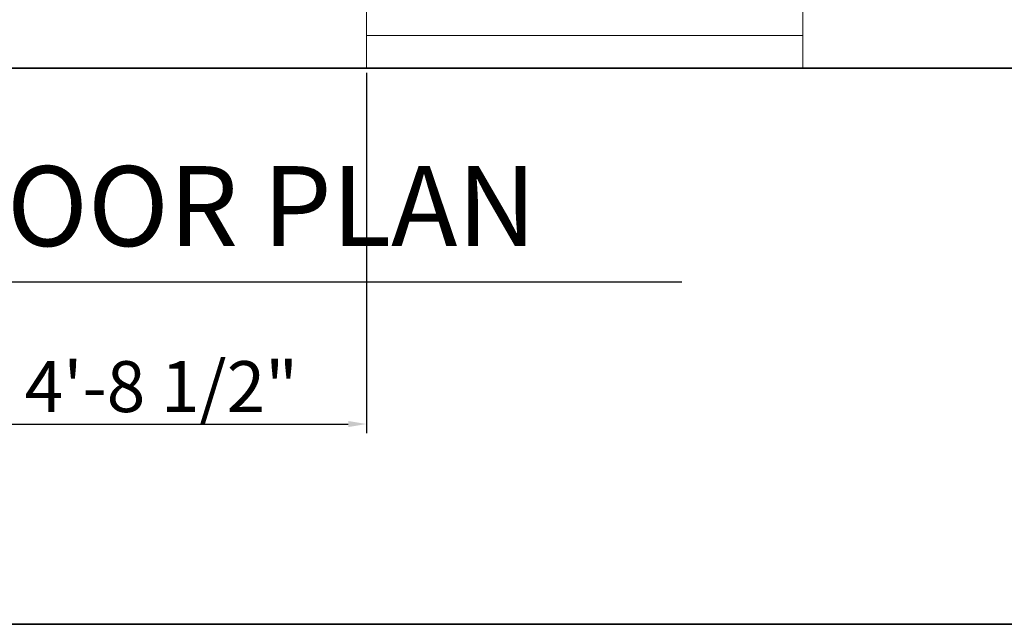
# Model space of a CAD drawing. Units: inches. Extents: x 1484 to 2008, y 1843 to 2590.
# Tile 2 of 21: x 1756 to 1891, y 1843 to 1926. Entities that reach past the tile are written whole.
import ezdxf

# ---------------------------------------------------------------- set-up
doc = ezdxf.new("R2010")
doc.units = ezdxf.units.IN
for name, color, linetype, lineweight in [('A-ANNO-DIMS', 2, 'Continuous', 18), ('A-ANNO-TEXT', 7, 'Continuous', 25), ('A-ANNO-TTLB', 7, 'Continuous', 35), ('A-GLAZ', 4, 'Continuous', 18), ('A-WALL', 7, 'Continuous', 35)]:
    doc.layers.add(name, color=color, linetype=linetype, lineweight=lineweight)
doc.styles.get("Standard").update_dxf_attribs({"font": 'arial.ttf'})
doc.dimstyles.new('ISO-25', dxfattribs={"dimtxt": 7, "dimasz": 2.5, "dimexe": 1.25, "dimexo": 0.625, "dimtad": 1, "dimdec": 0, "dimlunit": 3, "dimtxsty": 'Standard', "dimcen": 2.5, "dimadec": 0, "dimazin": 0, "dimtfac": 1, "dimtdec": 0, "dimtmove": 0, "dimatfit": 3, "dimfxl": 1, "dimarcsym": 0})

# ---------------------------------------------------------------- blocks, each defined once
blk = doc.blocks.new('WIN-60IN')
for p, q in [((0, 4.5), (0, -4.5)), ((60, 0), (60, 4.5)), ((60, 4.5), (60, -4.5)), ((0, -4.5), (0, 0)), ((0, 0), (60, 0))]:
    blk.add_line(p, q)
blk = doc.blocks.new('*D23')
at = {"layer": 'A-ANNO-DIMS', "color": 0, "lineweight": -2, "transparency": 16777216}
for p, q in [((1746.84, 1919.18), (1746.84, 1869.63)), ((1803.22, 1919.18), (1803.22, 1869.63)), ((1749.34, 1870.88), (1800.72, 1870.88))]:
    blk.add_line(p, q, dxfattribs=at)
at = {"layer": 'A-ANNO-DIMS', "color": 0, "transparency": 16777216}
for points in [[(1749.34, 1871.3), (1749.34, 1870.46), (1746.84, 1870.88)], [(1800.72, 1871.3), (1800.72, 1870.46), (1803.22, 1870.88)]]:
    blk.add_solid(points, dxfattribs=at)
at = {"layer": 'Defpoints', "color": 0, "transparency": 16777216}
for p in [(1746.84, 1919.8), (1803.22, 1919.8), (1803.22, 1870.88)]:
    blk.add_point(p, dxfattribs=at)
at = {"layer": 'A-ANNO-DIMS', "color": 0, "transparency": 16777216, "insert": (1775.03, 1875.12), "char_height": 7, "attachment_point": 5}
blk.add_mtext('4\'-8 1/2"', dxfattribs=at)

msp = doc.modelspace()

# ---------------------------------------------------------------- linework, layer by layer
at = {"layer": 'A-ANNO-TEXT'}
msp.add_line((1660.24, 1890.43), (1846.57, 1890.43), dxfattribs=at)
at = {"layer": 'A-ANNO-TTLB'}
msp.add_lwpolyline([(1484.04, 2590.09), (1989.53, 2590.09), (1989.53, 1843.34), (1484.04, 1843.34)], close=True, dxfattribs=at)
at = {"layer": 'A-WALL'}
msp.add_line((1686.99, 1919.8), (1899.92, 1919.8), dxfattribs=at)

# ---------------------------------------------------------------- block references
at = {"layer": 'A-GLAZ', "rotation": 180}
msp.add_blockref('WIN-60IN', (1863.22, 1924.3), dxfattribs=at)

# ---------------------------------------------------------------- texts
at = {"layer": 'A-ANNO-TEXT', "insert": (1671, 1906.35), "char_height": 11, "attachment_point": 1}
msp.add_mtext_dynamic_manual_height_columns('GROUND FLOOR PLAN', width=211.2221, gutter_width=12.5, heights=[0], dxfattribs=at)

# ---------------------------------------------------------------- dimensions: what is measured, and where the dimension line sits
at = {"layer": 'A-ANNO-DIMS'}
dim = msp.add_linear_dim(base=(1803.22, 1870.88), p1=(1746.84, 1919.8), p2=(1803.22, 1919.8), dimstyle='ISO-25', override={"dimdec": 1, "dimlfac": 1, "dimrnd": 0, "dimzin": 1, "dimdsep": 46, "dimlunit": 4, "dimfrac": 2}, dxfattribs=at)
dim.commit()
dim.dimension.update_dxf_attribs({"geometry": '*D23', "text_midpoint": (1775.03, 1875.12)})

doc.saveas('drawing.dxf')
